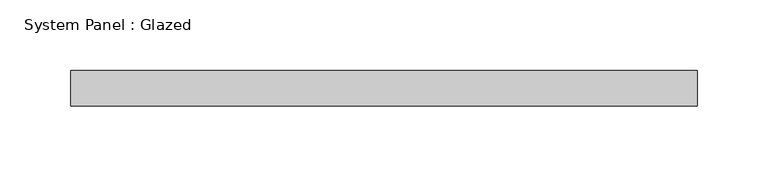
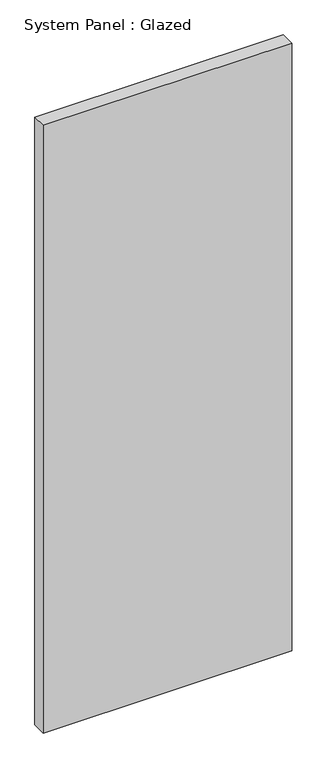
"""IFC4 building model written with IfcOpenShell, lengths in millimetres: plate geometry, System Panel : Glazed."""

from ifc_helpers import new_model, si_unit, origin, origin_with_axes, place, context, project, spatial, polyline, outline, extrude, source, transform, mapped, element, save


def system_panel_glazed_ad29da2a(model_context):
    return source(origin(), model_context, "Body", "SweptSolid", [
        extrude(outline(polyline([(222.25, 19.05), (-222.25, 19.05), (-222.25, 44.45), (222.25, 44.45), (222.25, 19.05)])), origin_with_axes(), (0.0, 0.0, 1.0), 1149.35),
    ])


if __name__ == "__main__":
    model = new_model("IFC4")
    model_context = context("Model", 3, world=origin())
    ifc_project = project(units=[si_unit("LENGTHUNIT", "METRE", prefix="MILLI")], contexts=[model_context])
    site = spatial("IfcSite", under=ifc_project)
    building = spatial("IfcBuilding", under=site)
    placement = place(None, origin())
    system_panel_glazed_shape = system_panel_glazed_ad29da2a(model_context)
    element("IfcPlate", 1, ObjectType="System Panel : Glazed", at=placement, inside=building, context=model_context, shape_type="MappedRepresentation", body=[
        mapped(system_panel_glazed_shape, transform((0.0, 0.0, 0.0), x_axis=(1.0, 0.0, 0.0), y_axis=(0.0, 1.0, 0.0), z_axis=(0.0, 0.0, 1.0))),
    ])
    save(model, "model.ifc")

# Revit data of these elements
# Type "System Panel : Glazed"
#   Construction Type Id = "GSP4R"
#   Analytic Construction = "1/8 in Pilkington single glazing"
#   Visual Light Transmittance = 0.9
#   Solar Heat Gain Coefficient = 0.86
#   Heat Transfer Coefficient (U) = 1.18115 BTU/(h·ft²·°F)
#   Define Thermal Properties by = 1
# Element 1 (IfcPlate, "System Panel : Glazed")
#   Materials on its faces: "Glass"
# Materials
#   "Glass": class "Glass", colour RGB 0 128 192, transparency 0.75, Description = "Soda Lime Glass", Cost = 0
